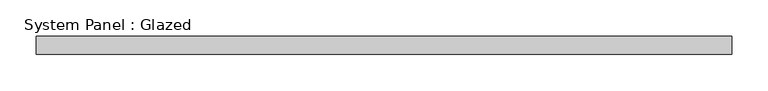
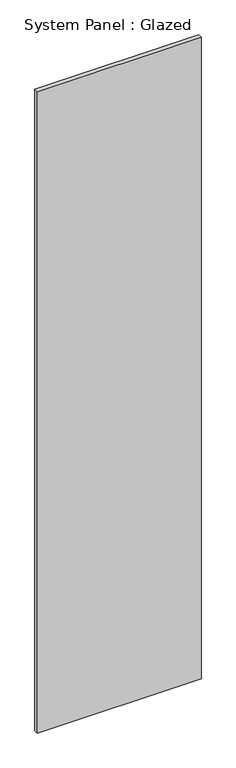
"""IFC4 building model written with IfcOpenShell, lengths in millimetres: plate geometry, System Panel : Glazed."""

from ifc_helpers import new_model, si_unit, origin, origin_with_axes, place, context, project, spatial, polyline, outline, extrude, source, transform, mapped, element, save


def system_panel_glazed_7dd01b14(model_context):
    return source(origin(), model_context, "Body", "SweptSolid", [
        extrude(outline(polyline([(482.6, 24.5), (-482.6, 24.5), (-482.6, 49.5), (482.6, 49.5), (482.6, 24.5)])), origin_with_axes(), (0.0, 0.0, 1.0), 4000.0),
    ])


if __name__ == "__main__":
    model = new_model("IFC4")
    model_context = context("Model", 3, world=origin())
    ifc_project = project(units=[si_unit("LENGTHUNIT", "METRE", prefix="MILLI")], contexts=[model_context])
    site = spatial("IfcSite", under=ifc_project)
    building = spatial("IfcBuilding", under=site)
    placement = place(None, origin())
    system_panel_glazed_shape = system_panel_glazed_7dd01b14(model_context)
    element("IfcPlate", 1, ObjectType="System Panel : Glazed", at=placement, inside=building, context=model_context, shape_type="MappedRepresentation", body=[
        mapped(system_panel_glazed_shape, transform((0.0, 0.0, 0.0), x_axis=(1.0, 0.0, 0.0), y_axis=(0.0, 1.0, 0.0), z_axis=(0.0, 0.0, 1.0))),
    ])
    save(model, "model.ifc")

# Revit data of these elements
# Type "System Panel : Glazed"
#   Keynote = "H11"
#   Construction Type Id = "GSP4R"
#   Analytic Construction = "1/8 in Pilkington single glazing"
#   Visual Light Transmittance = 0.9
#   Solar Heat Gain Coefficient = 0.86
#   Heat Transfer Coefficient (U) = 6.7069 W/(m²·K)
#   Define Thermal Properties by = 1
# Element 1 (IfcPlate, "System Panel : Glazed")
#   Materials on its faces: "Glass"
# Materials
#   "Glass": class "Glass", colour RGB 0 128 192, transparency 0.9, Description = "Soda Lime Glass", Cost = 0
